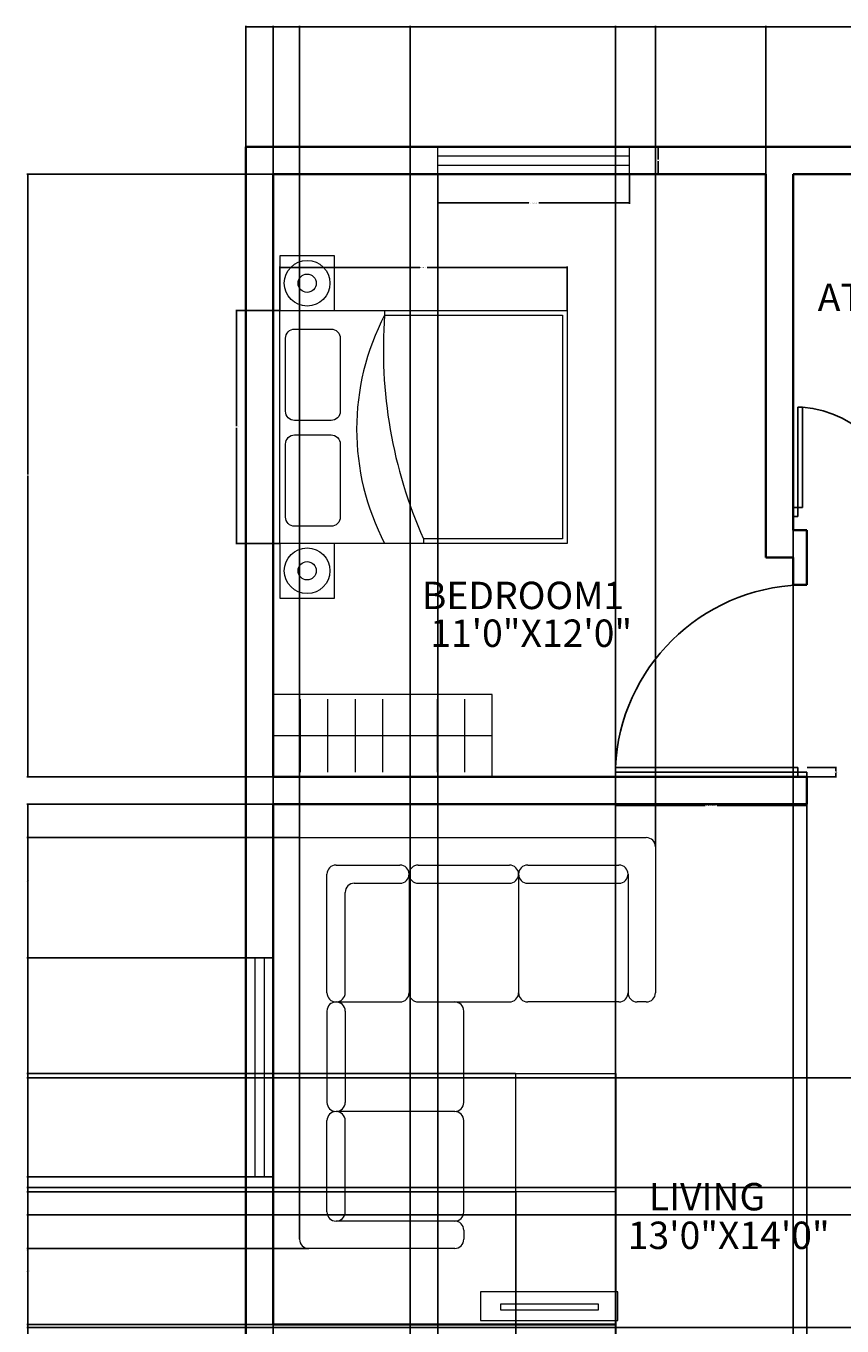
# Model space of a CAD drawing. Units: inches. Extents: x 2608 to 3003, y 1827 to 2396.
# Tile 3 of 5: x 2608 to 2787, y 2111 to 2396. Entities that reach past the tile are written whole.
import ezdxf

# ---------------------------------------------------------------- set-up
doc = ezdxf.new("R2010")
doc.units = ezdxf.units.IN
for name, color, linetype, lineweight in [('A-ANNO-DIMS', 2, 'Continuous', 18), ('A-AREA-IDEN', 7, 'Continuous', 25), ('A-DOOR', 50, 'Continuous', 25), ('A-EQPM', 213, 'Continuous', 18), ('A-FLOR-CASE', 213, 'Continuous', 18), ('A-FLOR-STRS', 111, 'Continuous', 25), ('A-FURN', 254, 'Continuous', 18), ('A-GLAZ', 40, 'Continuous', 18), ('A-WALL', 111, 'Continuous', 35)]:
    doc.layers.add(name, color=color, linetype=linetype, lineweight=lineweight)
doc.styles.get("Standard").update_dxf_attribs({"font": 'arial.ttf'})
doc.dimstyles.get("Standard").update_dxf_attribs({"dimtxt": 0.18, "dimasz": 0.18, "dimexe": 0.18, "dimexo": 0.0625, "dimgap": 0.09, "dimtad": 0, "dimtih": 1, "dimtoh": 1, "dimdec": 4, "dimzin": 0, "dimdsep": 46, "dimtxsty": 'Standard', "dimcen": 0.09, "dimadec": 0, "dimazin": 0, "dimtfac": 1, "dimtdec": 4, "dimtofl": 0, "dimtmove": 0, "dimatfit": 3, "dimfxl": 1, "dimtolj": 1, "dimtzin": 0, "dimarcsym": 0})

# ---------------------------------------------------------------- blocks, each defined once
blk = doc.blocks.new('BED-DOUBLE')
for p, q in [((22.99, 51), (22.99, 50)), ((22.99, 50), (61.99, 50)), ((61.99, 50), (61.99, 1)), ((61.99, 1), (31.5, 1)), ((31.5, 1), (31.5, 0))]:
    blk.add_line(p, q)
blk.add_lwpolyline([(0, 51), (63, 51), (63, 0), (0, 0)], close=True)
for points in [[(3.26, 46.94), (11.26, 46.94, -0.414214), (13.26, 44.94), (13.26, 28.94, -0.414214), (11.26, 26.94), (3.26, 26.94, -0.414214), (1.26, 28.94), (1.26, 44.94, -0.414214)], [(3.26, 23.76), (11.26, 23.76, -0.414214), (13.26, 21.76), (13.26, 5.76, -0.414214), (11.26, 3.76), (3.26, 3.76, -0.414214), (1.26, 5.76), (1.26, 21.76, -0.414214)]]:
    blk.add_lwpolyline(points, format="xyb", close=True)
for centre, radius, start, end in [((70.85, 25), 54, 152.4215, 207.5785), ((124.71, 42.43), 102, 175.743, 203.964)]:
    blk.add_arc(centre, radius, start, end)
blk = doc.blocks.new('NIGHTSTAND-LAMP')
blk.add_lwpolyline([(0, 0), (12, 0), (12, 12), (0, 12)], close=True)
for radius in [5, 2]:
    blk.add_circle((6, 6), radius)
blk = doc.blocks.new('WARDROBE-48')
for p, q in [((48, 18), (0, 18)), ((0, 18), (0, 0)), ((48, 0), (48, 18)), ((6, 1), (6, 17)), ((12, 1), (12, 17)), ((18, 1), (18, 17)), ((24, 1), (24, 17)), ((30, 1), (30, 17)), ((36, 1), (36, 17)), ((42, 1), (42, 17)), ((0, 9), (48, 9)), ((0, 0), (48, 0))]:
    blk.add_line(p, q)
blk = doc.blocks.new('WIN-42')
for p, q in [((0, 0), (0, 6)), ((42, 0), (42, 6)), ((0, 4), (42, 4)), ((0, 2), (42, 2))]:
    blk.add_line(p, q)
blk = doc.blocks.new('DOOR-LEAF-42')
for p, q in [((0, 1), (0, 2)), ((0, 2), (40, 2)), ((42, 1), (0, 1)), ((40, 2), (40, 0)), ((42, 0), (42, 1))]:
    blk.add_line(p, q)
blk = doc.blocks.new('*D14')
at = {"layer": 'A-ANNO-DIMS', "color": 0, "lineweight": -2, "transparency": 16777216}
for p, q in [((2663.35, 2333.66), (2663.35, 2343.23)), ((2663.53, 2343.05), (2694.03, 2343.05)), ((2726.17, 2343.05), (2695.67, 2343.05)), ((2726.35, 2333.66), (2726.35, 2343.23))]:
    blk.add_line(p, q, dxfattribs=at)
at = {"layer": 'A-ANNO-DIMS', "color": 0, "transparency": 16777216}
for points in [[(2663.53, 2343.08), (2663.53, 2343.02), (2663.35, 2343.05)], [(2726.17, 2343.08), (2726.17, 2343.02), (2726.35, 2343.05)]]:
    blk.add_solid(points, dxfattribs=at)
at = {"layer": 'Defpoints', "color": 0, "transparency": 16777216}
for p in [(2726.35, 2343.05), (2663.35, 2333.6), (2726.35, 2333.6)]:
    blk.add_point(p, dxfattribs=at)
at = {"layer": 'A-ANNO-DIMS', "color": 0, "transparency": 16777216, "insert": (2694.85, 2343.05), "char_height": 0.18, "attachment_point": 5}
blk.add_mtext('\\A1;BED 63 TYP.', dxfattribs=at)
blk = doc.blocks.new('*D15')
at = {"layer": 'A-ANNO-DIMS', "color": 0, "lineweight": -2, "transparency": 16777216}
for p, q in [((2663.29, 2333.6), (2653.72, 2333.6)), ((2653.9, 2333.42), (2653.9, 2308.28)), ((2653.9, 2282.78), (2653.9, 2307.92)), ((2663.29, 2282.6), (2653.72, 2282.6))]:
    blk.add_line(p, q, dxfattribs=at)
at = {"layer": 'A-ANNO-DIMS', "color": 0, "transparency": 16777216}
for points in [[(2653.87, 2333.42), (2653.93, 2333.42), (2653.9, 2333.6)], [(2653.87, 2282.78), (2653.93, 2282.78), (2653.9, 2282.6)]]:
    blk.add_solid(points, dxfattribs=at)
at = {"layer": 'Defpoints', "color": 0, "transparency": 16777216}
for p in [(2653.9, 2333.6), (2663.35, 2333.6), (2663.35, 2282.6)]:
    blk.add_point(p, dxfattribs=at)
at = {"layer": 'A-ANNO-DIMS', "color": 0, "transparency": 16777216, "insert": (2653.9, 2308.1), "char_height": 0.18, "attachment_point": 5}
blk.add_mtext('\\A1;51 TYP.', dxfattribs=at)
blk = doc.blocks.new('*D22')
at = {"layer": 'A-ANNO-DIMS', "color": 0, "lineweight": -2, "transparency": 16777216}
for p, q in [((2698.03, 2363.43), (2698.03, 2357.01)), ((2740.03, 2363.43), (2740.03, 2357.01)), ((2698.21, 2357.19), (2717.91, 2357.19)), ((2739.85, 2357.19), (2720.15, 2357.19))]:
    blk.add_line(p, q, dxfattribs=at)
at = {"layer": 'A-ANNO-DIMS', "color": 0, "transparency": 16777216}
for points in [[(2698.21, 2357.22), (2698.21, 2357.16), (2698.03, 2357.19)], [(2739.85, 2357.22), (2739.85, 2357.16), (2740.03, 2357.19)]]:
    blk.add_solid(points, dxfattribs=at)
at = {"layer": 'Defpoints', "color": 0, "transparency": 16777216}
for p in [(2698.03, 2363.49), (2740.03, 2363.49), (2740.03, 2357.19)]:
    blk.add_point(p, dxfattribs=at)
at = {"layer": 'A-ANNO-DIMS', "color": 0, "transparency": 16777216, "insert": (2719.03, 2357.19), "char_height": 0.18, "attachment_point": 5}
blk.add_mtext('\\A1;WINDOW 42 TYP.', dxfattribs=at)
blk = doc.blocks.new('*D23')
at = {"layer": 'A-ANNO-DIMS', "color": 0, "lineweight": -2, "transparency": 16777216}
for p, q in [((2740.09, 2369.49), (2746.51, 2369.49)), ((2746.33, 2369.31), (2746.33, 2366.67)), ((2746.33, 2363.67), (2746.33, 2366.31)), ((2740.09, 2363.49), (2746.51, 2363.49))]:
    blk.add_line(p, q, dxfattribs=at)
at = {"layer": 'A-ANNO-DIMS', "color": 0, "transparency": 16777216}
for points in [[(2746.3, 2369.31), (2746.36, 2369.31), (2746.33, 2369.49)], [(2746.3, 2363.67), (2746.36, 2363.67), (2746.33, 2363.49)]]:
    blk.add_solid(points, dxfattribs=at)
at = {"layer": 'Defpoints', "color": 0, "transparency": 16777216}
for p in [(2740.03, 2369.49), (2746.33, 2369.49), (2740.03, 2363.49)]:
    blk.add_point(p, dxfattribs=at)
at = {"layer": 'A-ANNO-DIMS', "color": 0, "transparency": 16777216, "insert": (2746.33, 2366.49), "char_height": 0.18, "attachment_point": 5}
blk.add_mtext('\\A1;6 TYP.', dxfattribs=at)
blk = doc.blocks.new('*D24')
at = {"layer": 'A-ANNO-DIMS', "color": 0, "lineweight": -2, "transparency": 16777216}
for p, q in [((2736.92, 2231.43), (2736.92, 2225.01)), ((2778.92, 2231.43), (2778.92, 2225.01)), ((2737.1, 2225.19), (2756.63, 2225.19)), ((2778.74, 2225.19), (2759.2, 2225.19))]:
    blk.add_line(p, q, dxfattribs=at)
at = {"layer": 'A-ANNO-DIMS', "color": 0, "transparency": 16777216}
for points in [[(2737.1, 2225.22), (2737.1, 2225.16), (2736.92, 2225.19)], [(2778.74, 2225.22), (2778.74, 2225.16), (2778.92, 2225.19)]]:
    blk.add_solid(points, dxfattribs=at)
at = {"layer": 'Defpoints', "color": 0, "transparency": 16777216}
for p in [(2736.92, 2231.49), (2778.92, 2231.49), (2778.92, 2225.19)]:
    blk.add_point(p, dxfattribs=at)
at = {"layer": 'A-ANNO-DIMS', "color": 0, "transparency": 16777216, "insert": (2757.92, 2225.19), "char_height": 0.18, "attachment_point": 5}
blk.add_mtext('\\A1;DOOR LEAF 42 TYP.', dxfattribs=at)
blk = doc.blocks.new('*D25')
at = {"layer": 'A-ANNO-DIMS', "color": 0, "lineweight": -2, "transparency": 16777216}
for p, q in [((2778.98, 2233.49), (2785.4, 2233.49)), ((2785.22, 2233.31), (2785.22, 2232.67)), ((2778.98, 2231.49), (2785.4, 2231.49)), ((2785.22, 2231.67), (2785.22, 2232.31))]:
    blk.add_line(p, q, dxfattribs=at)
at = {"layer": 'A-ANNO-DIMS', "color": 0, "transparency": 16777216}
for points in [[(2785.19, 2233.31), (2785.25, 2233.31), (2785.22, 2233.49)], [(2785.19, 2231.67), (2785.25, 2231.67), (2785.22, 2231.49)]]:
    blk.add_solid(points, dxfattribs=at)
at = {"layer": 'Defpoints', "color": 0, "transparency": 16777216}
for p in [(2778.92, 2233.49), (2785.22, 2233.49), (2778.92, 2231.49)]:
    blk.add_point(p, dxfattribs=at)
at = {"layer": 'A-ANNO-DIMS', "color": 0, "transparency": 16777216, "insert": (2785.22, 2232.49), "char_height": 0.18, "attachment_point": 5}
blk.add_mtext('\\A1;2 TYP.', dxfattribs=at)
blk = doc.blocks.new('*D28')
at = {"layer": 'A-ANNO-DIMS', "color": 0, "lineweight": -2, "transparency": 16777216}
for p, q in [((2655.92, 2191.9), (2655.92, 2395.95)), ((2656.1, 2395.77), (2805.63, 2395.77)), ((2955.74, 2395.77), (2806.2, 2395.77)), ((2955.92, 2201.05), (2955.92, 2395.95))]:
    blk.add_line(p, q, dxfattribs=at)
at = {"layer": 'A-ANNO-DIMS', "color": 0, "transparency": 16777216}
for points in [[(2656.1, 2395.8), (2656.1, 2395.74), (2655.92, 2395.77)], [(2955.74, 2395.8), (2955.74, 2395.74), (2955.92, 2395.77)]]:
    blk.add_solid(points, dxfattribs=at)
at = {"layer": 'Defpoints', "color": 0, "transparency": 16777216}
for p in [(2955.92, 2395.77), (2955.92, 2200.98), (2655.92, 2191.84)]:
    blk.add_point(p, dxfattribs=at)
at = {"layer": 'A-ANNO-DIMS', "color": 0, "transparency": 16777216, "insert": (2805.92, 2395.77), "char_height": 0.18, "attachment_point": 5}
blk.add_mtext('\\A1;300', dxfattribs=at)
blk = doc.blocks.new('*D35')
at = {"layer": 'A-ANNO-DIMS', "color": 0, "lineweight": -2, "transparency": 16777216}
for p, q in [((2661.85, 2143.84), (2607.92, 2143.84)), ((2608.1, 2143.66), (2608.1, 2127.85)), ((2608.1, 2111.67), (2608.1, 2127.48)), ((2661.85, 2111.49), (2607.92, 2111.49))]:
    blk.add_line(p, q, dxfattribs=at)
at = {"layer": 'A-ANNO-DIMS', "color": 0, "transparency": 16777216}
for points in [[(2608.07, 2143.66), (2608.13, 2143.66), (2608.1, 2143.84)], [(2608.07, 2111.67), (2608.13, 2111.67), (2608.1, 2111.49)]]:
    blk.add_solid(points, dxfattribs=at)
at = {"layer": 'Defpoints', "color": 0, "transparency": 16777216}
for p in [(2608.1, 2143.84), (2661.92, 2143.84), (2661.92, 2111.49)]:
    blk.add_point(p, dxfattribs=at)
at = {"layer": 'A-ANNO-DIMS', "color": 0, "transparency": 16777216, "insert": (2608.1, 2127.66), "char_height": 0.18, "attachment_point": 5}
blk.add_mtext('\\A1;32.35', dxfattribs=at)
blk = doc.blocks.new('*D36')
at = {"layer": 'A-ANNO-DIMS', "color": 0, "lineweight": -2, "transparency": 16777216}
for p, q in [((2655.85, 2191.84), (2607.92, 2191.84)), ((2608.1, 2191.66), (2608.1, 2168.02)), ((2608.1, 2144.02), (2608.1, 2167.66)), ((2655.85, 2143.84), (2607.92, 2143.84))]:
    blk.add_line(p, q, dxfattribs=at)
at = {"layer": 'A-ANNO-DIMS', "color": 0, "transparency": 16777216}
for points in [[(2608.07, 2191.66), (2608.13, 2191.66), (2608.1, 2191.84)], [(2608.07, 2144.02), (2608.13, 2144.02), (2608.1, 2143.84)]]:
    blk.add_solid(points, dxfattribs=at)
at = {"layer": 'Defpoints', "color": 0, "transparency": 16777216}
for p in [(2608.1, 2191.84), (2655.92, 2191.84), (2655.92, 2143.84)]:
    blk.add_point(p, dxfattribs=at)
at = {"layer": 'A-ANNO-DIMS', "color": 0, "transparency": 16777216, "insert": (2608.1, 2167.84), "char_height": 0.18, "attachment_point": 5}
blk.add_mtext('\\A1;48', dxfattribs=at)
blk = doc.blocks.new('*D37')
at = {"layer": 'A-ANNO-DIMS', "color": 0, "lineweight": -2, "transparency": 16777216}
for p, q in [((2661.85, 2225.49), (2607.92, 2225.49)), ((2608.1, 2225.31), (2608.1, 2208.85)), ((2608.1, 2192.02), (2608.1, 2208.48)), ((2661.85, 2191.84), (2607.92, 2191.84))]:
    blk.add_line(p, q, dxfattribs=at)
at = {"layer": 'A-ANNO-DIMS', "color": 0, "transparency": 16777216}
for points in [[(2608.07, 2225.31), (2608.13, 2225.31), (2608.1, 2225.49)], [(2608.07, 2192.02), (2608.13, 2192.02), (2608.1, 2191.84)]]:
    blk.add_solid(points, dxfattribs=at)
at = {"layer": 'Defpoints', "color": 0, "transparency": 16777216}
for p in [(2608.1, 2225.49), (2661.92, 2225.49), (2661.92, 2191.84)]:
    blk.add_point(p, dxfattribs=at)
at = {"layer": 'A-ANNO-DIMS', "color": 0, "transparency": 16777216, "insert": (2608.1, 2208.66), "char_height": 0.18, "attachment_point": 5}
blk.add_mtext('\\A1;33.65', dxfattribs=at)
blk = doc.blocks.new('*D38')
at = {"layer": 'A-ANNO-DIMS', "color": 0, "lineweight": -2, "transparency": 16777216}
for p, q in [((2661.92, 2363.55), (2661.92, 2395.95)), ((2662.1, 2395.77), (2715.63, 2395.77)), ((2769.74, 2395.77), (2716.2, 2395.77)), ((2769.92, 2363.55), (2769.92, 2395.95))]:
    blk.add_line(p, q, dxfattribs=at)
at = {"layer": 'A-ANNO-DIMS', "color": 0, "transparency": 16777216}
for points in [[(2662.1, 2395.8), (2662.1, 2395.74), (2661.92, 2395.77)], [(2769.74, 2395.8), (2769.74, 2395.74), (2769.92, 2395.77)]]:
    blk.add_solid(points, dxfattribs=at)
at = {"layer": 'Defpoints', "color": 0, "transparency": 16777216}
for p in [(2769.92, 2395.77), (2661.92, 2363.49), (2769.92, 2363.49)]:
    blk.add_point(p, dxfattribs=at)
at = {"layer": 'A-ANNO-DIMS', "color": 0, "transparency": 16777216, "insert": (2715.92, 2395.77), "char_height": 0.18, "attachment_point": 5}
blk.add_mtext('\\A1;108', dxfattribs=at)
blk = doc.blocks.new('*D40')
at = {"layer": 'A-ANNO-DIMS', "color": 0, "lineweight": -2, "transparency": 16777216}
for p, q in [((2661.85, 2363.49), (2607.92, 2363.49)), ((2608.1, 2363.31), (2608.1, 2297.67)), ((2608.1, 2231.67), (2608.1, 2297.31)), ((2661.85, 2231.49), (2607.92, 2231.49))]:
    blk.add_line(p, q, dxfattribs=at)
at = {"layer": 'A-ANNO-DIMS', "color": 0, "transparency": 16777216}
for points in [[(2608.07, 2363.31), (2608.13, 2363.31), (2608.1, 2363.49)], [(2608.07, 2231.67), (2608.13, 2231.67), (2608.1, 2231.49)]]:
    blk.add_solid(points, dxfattribs=at)
at = {"layer": 'Defpoints', "color": 0, "transparency": 16777216}
for p in [(2608.1, 2363.49), (2661.92, 2363.49), (2661.92, 2231.49)]:
    blk.add_point(p, dxfattribs=at)
at = {"layer": 'A-ANNO-DIMS', "color": 0, "transparency": 16777216, "insert": (2608.1, 2297.49), "char_height": 0.18, "attachment_point": 5}
blk.add_mtext('\\A1;132', dxfattribs=at)
blk = doc.blocks.new('*D42')
at = {"layer": 'A-ANNO-DIMS', "color": 0, "lineweight": -2, "transparency": 16777216}
for p, q in [((2775.92, 2285.43), (2775.92, 1827.03)), ((2799.92, 2285.43), (2799.92, 1827.03)), ((2776.1, 1827.21), (2787.7, 1827.21)), ((2799.74, 1827.21), (2788.14, 1827.21))]:
    blk.add_line(p, q, dxfattribs=at)
at = {"layer": 'A-ANNO-DIMS', "color": 0, "transparency": 16777216}
for points in [[(2776.1, 1827.24), (2776.1, 1827.18), (2775.92, 1827.21)], [(2799.74, 1827.24), (2799.74, 1827.18), (2799.92, 1827.21)]]:
    blk.add_solid(points, dxfattribs=at)
at = {"layer": 'Defpoints', "color": 0, "transparency": 16777216}
for p in [(2775.92, 2285.49), (2799.92, 2285.49), (2799.92, 1827.21)]:
    blk.add_point(p, dxfattribs=at)
at = {"layer": 'A-ANNO-DIMS', "color": 0, "transparency": 16777216, "insert": (2787.92, 1827.21), "char_height": 0.18, "attachment_point": 5}
blk.add_mtext('\\A1;24', dxfattribs=at)
blk = doc.blocks.new('*D43')
at = {"layer": 'A-ANNO-DIMS', "color": 0, "lineweight": -2, "transparency": 16777216}
for p, q in [((2661.92, 2363.43), (2661.92, 1827.03)), ((2698.03, 2363.43), (2698.03, 1827.03)), ((2662.1, 1827.21), (2679.51, 1827.21)), ((2697.85, 1827.21), (2680.44, 1827.21))]:
    blk.add_line(p, q, dxfattribs=at)
at = {"layer": 'A-ANNO-DIMS', "color": 0, "transparency": 16777216}
for points in [[(2662.1, 1827.24), (2662.1, 1827.18), (2661.92, 1827.21)], [(2697.85, 1827.24), (2697.85, 1827.18), (2698.03, 1827.21)]]:
    blk.add_solid(points, dxfattribs=at)
at = {"layer": 'Defpoints', "color": 0, "transparency": 16777216}
for p in [(2661.92, 2363.49), (2698.03, 2363.49), (2698.03, 1827.21)]:
    blk.add_point(p, dxfattribs=at)
at = {"layer": 'A-ANNO-DIMS', "color": 0, "transparency": 16777216, "insert": (2679.97, 1827.21), "char_height": 0.18, "attachment_point": 5}
blk.add_mtext('\\A1;36.116', dxfattribs=at)
blk = doc.blocks.new('*D44')
at = {"layer": 'A-ANNO-DIMS', "color": 0, "lineweight": -2, "transparency": 16777216}
for p, q in [((2775.92, 2363.43), (2775.92, 1827.03)), ((2795.68, 2363.43), (2795.68, 1827.03)), ((2776.1, 1827.21), (2785.34, 1827.21)), ((2795.5, 1827.21), (2786.25, 1827.21))]:
    blk.add_line(p, q, dxfattribs=at)
at = {"layer": 'A-ANNO-DIMS', "color": 0, "transparency": 16777216}
for points in [[(2776.1, 1827.24), (2776.1, 1827.18), (2775.92, 1827.21)], [(2795.5, 1827.24), (2795.5, 1827.18), (2795.68, 1827.21)]]:
    blk.add_solid(points, dxfattribs=at)
at = {"layer": 'Defpoints', "color": 0, "transparency": 16777216}
for p in [(2775.92, 2363.49), (2795.68, 2363.49), (2795.68, 1827.21)]:
    blk.add_point(p, dxfattribs=at)
at = {"layer": 'A-ANNO-DIMS', "color": 0, "transparency": 16777216, "insert": (2785.8, 1827.21), "char_height": 0.18, "attachment_point": 5}
blk.add_mtext('\\A1;19.766', dxfattribs=at)
blk = doc.blocks.new('*D47')
at = {"layer": 'A-ANNO-DIMS', "color": 0, "lineweight": -2, "transparency": 16777216}
for p, q in [((2778.92, 2225.43), (2778.92, 1827.03)), ((2835.92, 2225.43), (2835.92, 1827.03)), ((2779.1, 1827.21), (2807.2, 1827.21)), ((2835.74, 1827.21), (2807.63, 1827.21))]:
    blk.add_line(p, q, dxfattribs=at)
at = {"layer": 'A-ANNO-DIMS', "color": 0, "transparency": 16777216}
for points in [[(2779.1, 1827.24), (2779.1, 1827.18), (2778.92, 1827.21)], [(2835.74, 1827.24), (2835.74, 1827.18), (2835.92, 1827.21)]]:
    blk.add_solid(points, dxfattribs=at)
at = {"layer": 'Defpoints', "color": 0, "transparency": 16777216}
for p in [(2778.92, 2225.49), (2835.92, 2225.49), (2835.92, 1827.21)]:
    blk.add_point(p, dxfattribs=at)
at = {"layer": 'A-ANNO-DIMS', "color": 0, "transparency": 16777216, "insert": (2807.42, 1827.21), "char_height": 0.18, "attachment_point": 5}
blk.add_mtext('\\A1;57', dxfattribs=at)
blk = doc.blocks.new('*D48')
at = {"layer": 'A-ANNO-DIMS', "color": 0, "lineweight": -2, "transparency": 16777216}
for p, q in [((2889.85, 2165.49), (2607.92, 2165.49)), ((2608.1, 2165.31), (2608.1, 2153.67)), ((2608.1, 2141.67), (2608.1, 2153.31)), ((2889.85, 2141.49), (2607.92, 2141.49))]:
    blk.add_line(p, q, dxfattribs=at)
at = {"layer": 'A-ANNO-DIMS', "color": 0, "transparency": 16777216}
for points in [[(2608.07, 2165.31), (2608.13, 2165.31), (2608.1, 2165.49)], [(2608.07, 2141.67), (2608.13, 2141.67), (2608.1, 2141.49)]]:
    blk.add_solid(points, dxfattribs=at)
at = {"layer": 'Defpoints', "color": 0, "transparency": 16777216}
for p in [(2608.1, 2165.49), (2889.92, 2165.49), (2889.92, 2141.49)]:
    blk.add_point(p, dxfattribs=at)
at = {"layer": 'A-ANNO-DIMS', "color": 0, "transparency": 16777216, "insert": (2608.1, 2153.49), "char_height": 0.18, "attachment_point": 5}
blk.add_mtext('\\A1;24', dxfattribs=at)
blk = doc.blocks.new('*D55')
at = {"layer": 'A-ANNO-DIMS', "color": 0, "lineweight": -2, "transparency": 16777216}
for p, q in [((2847.85, 2135.49), (2607.92, 2135.49)), ((2608.1, 2135.31), (2608.1, 2122.17)), ((2608.1, 2108.67), (2608.1, 2121.81)), ((2853.85, 2108.49), (2607.92, 2108.49))]:
    blk.add_line(p, q, dxfattribs=at)
at = {"layer": 'A-ANNO-DIMS', "color": 0, "transparency": 16777216}
for points in [[(2608.07, 2135.31), (2608.13, 2135.31), (2608.1, 2135.49)], [(2608.07, 2108.67), (2608.13, 2108.67), (2608.1, 2108.49)]]:
    blk.add_solid(points, dxfattribs=at)
at = {"layer": 'Defpoints', "color": 0, "transparency": 16777216}
for p in [(2608.1, 2135.49), (2847.92, 2135.49), (2853.92, 2108.49)]:
    blk.add_point(p, dxfattribs=at)
at = {"layer": 'A-ANNO-DIMS', "color": 0, "transparency": 16777216, "insert": (2608.1, 2121.99), "char_height": 0.18, "attachment_point": 5}
blk.add_mtext('\\A1;27', dxfattribs=at)
blk = doc.blocks.new('*D62')
at = {"layer": 'A-ANNO-DIMS', "color": 0, "lineweight": -2, "transparency": 16777216}
for p, q in [((2925.85, 2135.49), (2607.92, 2135.49)), ((2608.1, 2135.31), (2608.1, 2123.33)), ((2608.1, 2110.99), (2608.1, 2122.97)), ((2928.1, 2110.81), (2607.92, 2110.81))]:
    blk.add_line(p, q, dxfattribs=at)
at = {"layer": 'A-ANNO-DIMS', "color": 0, "transparency": 16777216}
for points in [[(2608.07, 2135.31), (2608.13, 2135.31), (2608.1, 2135.49)], [(2608.07, 2110.99), (2608.13, 2110.99), (2608.1, 2110.81)]]:
    blk.add_solid(points, dxfattribs=at)
at = {"layer": 'Defpoints', "color": 0, "transparency": 16777216}
for p in [(2925.92, 2135.49), (2608.1, 2110.81), (2928.16, 2110.81)]:
    blk.add_point(p, dxfattribs=at)
at = {"layer": 'A-ANNO-DIMS', "color": 0, "transparency": 16777216, "insert": (2608.1, 2123.15), "char_height": 0.18, "attachment_point": 5}
blk.add_mtext('\\A1;24.675', dxfattribs=at)
blk = doc.blocks.new('*D69')
at = {"layer": 'A-ANNO-DIMS', "color": 0, "lineweight": -2, "transparency": 16777216}
for p, q in [((2691.92, 2105.55), (2691.92, 2395.95)), ((2692.1, 2395.77), (2714.19, 2395.77)), ((2736.74, 2395.77), (2714.64, 2395.77)), ((2736.92, 2105.55), (2736.92, 2395.95))]:
    blk.add_line(p, q, dxfattribs=at)
at = {"layer": 'A-ANNO-DIMS', "color": 0, "transparency": 16777216}
for points in [[(2692.1, 2395.8), (2692.1, 2395.74), (2691.92, 2395.77)], [(2736.74, 2395.8), (2736.74, 2395.74), (2736.92, 2395.77)]]:
    blk.add_solid(points, dxfattribs=at)
at = {"layer": 'Defpoints', "color": 0, "transparency": 16777216}
for p in [(2736.92, 2395.77), (2691.92, 2105.49), (2736.92, 2105.49)]:
    blk.add_point(p, dxfattribs=at)
at = {"layer": 'A-ANNO-DIMS', "color": 0, "transparency": 16777216, "insert": (2714.42, 2395.77), "char_height": 0.18, "attachment_point": 5}
blk.add_mtext('\\A1;45', dxfattribs=at)
blk = doc.blocks.new('*D72')
at = {"layer": 'A-ANNO-DIMS', "color": 0, "lineweight": -2, "transparency": 16777216}
for p, q in [((2715.11, 2140.45), (2715.11, 1827.03)), ((2737, 2140.45), (2737, 1827.03)), ((2715.29, 1827.21), (2725.66, 1827.21)), ((2736.82, 1827.21), (2726.45, 1827.21))]:
    blk.add_line(p, q, dxfattribs=at)
at = {"layer": 'A-ANNO-DIMS', "color": 0, "transparency": 16777216}
for points in [[(2715.29, 1827.24), (2715.29, 1827.18), (2715.11, 1827.21)], [(2736.82, 1827.24), (2736.82, 1827.18), (2737, 1827.21)]]:
    blk.add_solid(points, dxfattribs=at)
at = {"layer": 'Defpoints', "color": 0, "transparency": 16777216}
for p in [(2715.11, 2140.51), (2737, 2140.51), (2737, 1827.21)]:
    blk.add_point(p, dxfattribs=at)
at = {"layer": 'A-ANNO-DIMS', "color": 0, "transparency": 16777216, "insert": (2726.06, 1827.21), "char_height": 0.18, "attachment_point": 5}
blk.add_mtext('\\A1;21.89', dxfattribs=at)
blk = doc.blocks.new('*D73')
at = {"layer": 'A-ANNO-DIMS', "color": 0, "lineweight": -2, "transparency": 16777216}
for p, q in [((2715.05, 2166.47), (2607.92, 2166.47)), ((2608.1, 2166.29), (2608.1, 2153.67)), ((2608.1, 2140.69), (2608.1, 2153.31)), ((2715.05, 2140.51), (2607.92, 2140.51))]:
    blk.add_line(p, q, dxfattribs=at)
at = {"layer": 'A-ANNO-DIMS', "color": 0, "transparency": 16777216}
for points in [[(2608.07, 2166.29), (2608.13, 2166.29), (2608.1, 2166.47)], [(2608.07, 2140.69), (2608.13, 2140.69), (2608.1, 2140.51)]]:
    blk.add_solid(points, dxfattribs=at)
at = {"layer": 'Defpoints', "color": 0, "transparency": 16777216}
for p in [(2608.1, 2166.47), (2715.11, 2166.47), (2715.11, 2140.51)]:
    blk.add_point(p, dxfattribs=at)
at = {"layer": 'A-ANNO-DIMS', "color": 0, "transparency": 16777216, "insert": (2608.1, 2153.49), "char_height": 0.18, "attachment_point": 5}
blk.add_mtext('\\A1;25.96', dxfattribs=at)
blk = doc.blocks.new('*D74')
at = {"layer": 'A-ANNO-DIMS', "color": 0, "lineweight": -2, "transparency": 16777216}
for p, q in [((2667.69, 2130.21), (2667.69, 2395.95)), ((2667.87, 2395.77), (2706.47, 2395.77)), ((2745.51, 2395.77), (2706.91, 2395.77)), ((2745.69, 2216.21), (2745.69, 2395.95))]:
    blk.add_line(p, q, dxfattribs=at)
at = {"layer": 'A-ANNO-DIMS', "color": 0, "transparency": 16777216}
for points in [[(2667.87, 2395.8), (2667.87, 2395.74), (2667.69, 2395.77)], [(2745.51, 2395.8), (2745.51, 2395.74), (2745.69, 2395.77)]]:
    blk.add_solid(points, dxfattribs=at)
at = {"layer": 'Defpoints', "color": 0, "transparency": 16777216}
for p in [(2745.69, 2395.77), (2745.69, 2216.14), (2667.69, 2130.14)]:
    blk.add_point(p, dxfattribs=at)
at = {"layer": 'A-ANNO-DIMS', "color": 0, "transparency": 16777216, "insert": (2706.69, 2395.77), "char_height": 0.18, "attachment_point": 5}
blk.add_mtext('\\A1;78', dxfattribs=at)
blk = doc.blocks.new('*D75')
at = {"layer": 'A-ANNO-DIMS', "color": 0, "lineweight": -2, "transparency": 16777216}
for p, q in [((2667.63, 2218.14), (2607.92, 2218.14)), ((2608.1, 2217.96), (2608.1, 2173.32)), ((2608.1, 2128.32), (2608.1, 2172.96)), ((2669.63, 2128.14), (2607.92, 2128.14))]:
    blk.add_line(p, q, dxfattribs=at)
at = {"layer": 'A-ANNO-DIMS', "color": 0, "transparency": 16777216}
for points in [[(2608.07, 2217.96), (2608.13, 2217.96), (2608.1, 2218.14)], [(2608.07, 2128.32), (2608.13, 2128.32), (2608.1, 2128.14)]]:
    blk.add_solid(points, dxfattribs=at)
at = {"layer": 'Defpoints', "color": 0, "transparency": 16777216}
for p in [(2608.1, 2218.14), (2667.69, 2218.14), (2669.69, 2128.14)]:
    blk.add_point(p, dxfattribs=at)
at = {"layer": 'A-ANNO-DIMS', "color": 0, "transparency": 16777216, "insert": (2608.1, 2173.14), "char_height": 0.18, "attachment_point": 5}
blk.add_mtext('\\A1;90', dxfattribs=at)
blk = doc.blocks.new('*D76')
at = {"layer": 'A-ANNO-DIMS', "color": 0, "lineweight": -2, "transparency": 16777216}
for p, q in [((2813.16, 2112.32), (2794.82, 2095.3)), ((2813.34, 2112.32), (2813.16, 2112.32)), ((2763.83, 2066.6), (2764.01, 2066.6)), ((2763.92, 2066.51), (2763.92, 2066.69))]:
    blk.add_line(p, q, dxfattribs=at)
at = {"layer": 'A-ANNO-DIMS', "color": 0, "transparency": 16777216}
blk.add_solid([(2794.8, 2095.32), (2794.85, 2095.28), (2794.69, 2095.18)], dxfattribs=at)
at = {"layer": 'Defpoints', "color": 0, "transparency": 16777216}
for p in [(2794.69, 2095.18), (2763.92, 2066.6)]:
    blk.add_point(p, dxfattribs=at)
at = {"layer": 'A-ANNO-DIMS', "color": 0, "transparency": 16777216, "insert": (2813.64, 2112.32), "char_height": 0.18, "attachment_point": 5}
blk.add_mtext('\\A1;R42', dxfattribs=at)

msp = doc.modelspace()

# ---------------------------------------------------------------- linework, layer by layer
at = {"layer": 'A-DOOR'}
for p, q in [((2776.9155, 2288.4603), (2776.9155, 2312.4603)), ((2776.9155, 2312.4603), (2777.9155, 2312.4603)), ((2777.9155, 2312.4603), (2777.9155, 2290.4603)), ((2777.9155, 2290.4603), (2775.9155, 2290.4603)), ((2775.9155, 2288.4603), (2776.9155, 2288.4603))]:
    msp.add_line(p, q, dxfattribs=at)
for centre, radius, start, end in [((2775.9156, 2288.5438), 24, 359.870639, 85.219955), ((2778.8691, 2231.5148), 42, 91.983302, 177.304959)]:
    msp.add_arc(centre, radius, start, end, dxfattribs=at)
at = {"layer": 'A-EQPM'}
for points in [[(2707.3148, 2112.3224), (2737.4539, 2112.3224), (2737.4539, 2118.6043), (2707.3148, 2118.6043)], [(2711.7858, 2115.998), (2733.1602, 2115.998), (2733.1602, 2114.593), (2711.7858, 2114.593)]]:
    msp.add_lwpolyline(points, close=True, dxfattribs=at)
at = {"layer": 'A-FLOR-CASE'}
msp.add_line((2661.9155, 2231.4896), (2661.9155, 2249.4896), dxfattribs=at)
at = {"layer": 'A-FLOR-STRS'}
msp.add_line((2736.9155, 2067.4896), (2736.9155, 2111.4896), dxfattribs=at)
at = {"layer": 'A-FURN'}
for p, q in [((2667.6933, 2218.1429), (2743.6933, 2218.1429)), ((2667.6933, 2182.1429), (2667.6933, 2218.1429)), ((2745.6933, 2216.1429), (2745.6933, 2184.1429)), ((2673.6933, 2184.1429), (2673.6933, 2210.1429)), ((2675.6933, 2212.1429), (2689.6933, 2212.1429)), ((2691.6933, 2210.1429), (2691.6933, 2210.1429)), ((2691.6933, 2210.1429), (2691.6933, 2210.1429)), ((2691.6933, 2210.1429), (2691.6933, 2184.1429)), ((2693.6933, 2212.1429), (2713.6933, 2212.1429)), ((2715.6933, 2210.1429), (2715.6933, 2210.1429)), ((2715.6933, 2210.1429), (2715.6933, 2210.1429)), ((2715.6933, 2210.1429), (2715.6933, 2184.1429)), ((2717.6933, 2212.1429), (2737.6933, 2212.1429)), ((2739.6933, 2210.1429), (2739.6933, 2210.1429)), ((2739.6933, 2210.1429), (2739.6933, 2184.1429)), ((2679.6933, 2208.1429), (2689.6933, 2208.1429)), ((2693.6933, 2208.1429), (2713.6933, 2208.1429)), ((2717.6933, 2208.1429), (2737.6933, 2208.1429)), ((2677.6933, 2184.1429), (2677.6933, 2206.1429)), ((2667.6933, 2130.1429), (2667.6933, 2182.1429)), ((2675.6933, 2182.1429), (2675.6933, 2182.1429)), ((2675.6933, 2182.1429), (2675.6933, 2182.1429)), ((2675.6933, 2182.1429), (2689.6933, 2182.1429)), ((2691.6933, 2184.1429), (2691.6933, 2184.1429)), ((2693.6933, 2182.1429), (2701.6933, 2182.1429)), ((2701.6933, 2182.1429), (2713.6933, 2182.1429)), ((2715.6933, 2184.1429), (2715.6933, 2184.1429)), ((2737.6933, 2182.1429), (2717.6933, 2182.1429)), ((2739.6933, 2184.1429), (2739.6933, 2184.1429)), ((2743.6933, 2182.1429), (2741.6933, 2182.1429)), ((2673.6933, 2180.1429), (2673.6933, 2160.1429)), ((2677.6933, 2180.1429), (2677.6933, 2160.1429)), ((2703.6933, 2160.1429), (2703.6933, 2180.1429)), ((2673.6933, 2136.1429), (2673.6933, 2156.1429)), ((2675.6933, 2158.1429), (2675.6933, 2158.1429)), ((2675.6933, 2158.1429), (2675.6933, 2158.1429)), ((2701.6933, 2158.1429), (2675.6933, 2158.1429)), ((2677.6933, 2136.1429), (2677.6933, 2156.1429)), ((2701.6933, 2158.1429), (2701.6933, 2158.1429)), ((2703.6933, 2136.1429), (2703.6933, 2156.1429)), ((2675.6933, 2134.1429), (2675.6933, 2134.1429)), ((2701.6933, 2134.1429), (2675.6933, 2134.1429)), ((2701.6933, 2134.1429), (2701.6933, 2134.1429)), ((2703.6933, 2132.1429), (2703.6933, 2130.1429)), ((2701.6933, 2128.1429), (2669.6933, 2128.1429))]:
    msp.add_line(p, q, dxfattribs=at)
msp.add_lwpolyline([(2715.1137, 2166.4712), (2737.0038, 2166.4712), (2737.0038, 2140.51), (2715.1137, 2140.51)], close=True, dxfattribs=at)
for centre, start, end in [((2743.6933, 2216.1429), 0, 90), ((2675.6933, 2210.1429), 90, 180), ((2689.6933, 2210.1429), 360, 90), ((2689.6933, 2210.1429), 270, 360), ((2693.6933, 2210.1429), 90, 180), ((2693.6933, 2210.1429), 180, 270), ((2713.6933, 2210.1429), 0, 90), ((2713.6933, 2210.1429), 270, 0), ((2717.6933, 2210.1429), 90, 180), ((2717.6933, 2210.1429), 180, 270), ((2737.6933, 2210.1429), 0, 90), ((2737.6933, 2210.1429), 270, 0), ((2679.6933, 2206.1429), 90, 180), ((2675.6933, 2184.1429), 180, 270), ((2675.6933, 2180.1429), 90, 180), ((2675.6933, 2184.1429), 270, 0), ((2675.6933, 2180.1429), 0, 90), ((2689.6933, 2184.1429), 270, 0), ((2693.6933, 2184.1429), 180, 270), ((2701.6933, 2180.1429), 0, 90), ((2713.6933, 2184.1429), 270, 0), ((2717.6933, 2184.1429), 180, 270), ((2737.6933, 2184.1429), 270, 0), ((2741.6933, 2184.1429), 180, 270), ((2743.6933, 2184.1429), 270, 0), ((2675.6933, 2160.1429), 180, 270), ((2675.6933, 2160.1429), 270, 0), ((2701.6933, 2160.1429), 270, 0), ((2675.6933, 2156.1429), 90, 180), ((2675.6933, 2156.1429), 0, 90), ((2701.6933, 2156.1429), 0, 90), ((2675.6933, 2136.1429), 180, 270), ((2675.6933, 2136.1429), 270, 0), ((2701.6933, 2136.1429), 270, 0), ((2701.6933, 2132.1429), 0, 90), ((2669.6933, 2130.1429), 180, 270), ((2701.6933, 2130.1429), 270, 0)]:
    msp.add_arc(centre, 2, start, end, dxfattribs=at)
at = {"layer": 'A-GLAZ'}
for p, q in [((2661.9155, 2191.8395), (2655.9155, 2191.8395)), ((2657.9155, 2191.8395), (2657.9155, 2143.8395)), ((2659.9155, 2191.8395), (2659.9155, 2143.8395)), ((2661.9155, 2143.8395), (2655.9155, 2143.8395))]:
    msp.add_line(p, q, dxfattribs=at)
at = {"layer": 'A-WALL'}
for p, q in [((2661.9155, 2363.4896), (2769.9155, 2363.4896)), ((2661.9155, 2231.4896), (2661.9155, 2363.4896)), ((2769.9155, 2279.4896), (2769.9155, 2363.4896)), ((2775.9155, 2285.4896), (2775.9155, 2363.4896)), ((2775.9155, 2363.4896), (2835.9155, 2363.4896)), ((2775.9155, 2285.4896), (2778.9155, 2285.4896)), ((2778.9155, 2273.4896), (2778.9155, 2285.4896)), ((2769.9155, 2279.4896), (2775.9155, 2279.4896)), ((2775.9155, 2273.4896), (2775.9155, 2279.4896)), ((2775.9155, 2273.4896), (2778.9155, 2273.4896)), ((2661.9155, 2231.4896), (2778.9155, 2231.4896)), ((2778.9155, 2225.4896), (2778.9155, 2231.4896)), ((2661.9155, 2225.4896), (2778.9155, 2225.4896)), ((2661.9155, 2111.4896), (2661.9155, 2225.4896)), ((2661.9155, 2111.4896), (2736.9155, 2111.4896))]:
    msp.add_line(p, q, dxfattribs=at)
msp.add_lwpolyline([(2655.9155, 2369.4896), (2955.9155, 2369.4896), (2955.9155, 1889.4896), (2655.9155, 1889.4896)], close=True, dxfattribs=at)

# ---------------------------------------------------------------- block references
at = {"layer": 'A-DOOR'}
msp.add_blockref('DOOR-LEAF-42', (2736.916, 2231.49), dxfattribs=at)
at = {"layer": 'A-FLOR-CASE'}
msp.add_blockref('WARDROBE-48', (2661.916, 2231.49), dxfattribs=at)
at = {"layer": 'A-FURN'}
for name, p in [('NIGHTSTAND-LAMP', (2663.348, 2333.601)), ('BED-DOUBLE', (2663.348, 2282.601))]:
    msp.add_blockref(name, p, dxfattribs=at)
at = {"layer": 'A-FURN', "rotation": 269.9999999999942}
msp.add_blockref('NIGHTSTAND-LAMP', (2663.3481, 2282.6011), dxfattribs=at)
at = {"layer": 'A-GLAZ'}
msp.add_blockref('WIN-42', (2698.032, 2363.49), dxfattribs=at)

# ---------------------------------------------------------------- texts
at = {"layer": 'A-AREA-IDEN'}
for tag, p in [('ATT.TOILET', (2781.2685, 2333.5052)), ('BEDROOM1', (2694.4884, 2268.2025)), ('11\'0"X12\'0"', (2696.3326, 2259.9258)), ('LIVING', (2744.2547, 2136.4817)), ('13\'0"X14\'0"', (2739.6279, 2128.0189))]:
    msp.add_attdef(tag, p, '', height=6, dxfattribs=at)

# ---------------------------------------------------------------- dimensions: what is measured, and where the dimension line sits
at = {"layer": 'A-ANNO-DIMS'}
for base, p1, p2, override, picture, middle in [((2955.9155, 2395.7696), (2655.9155, 2191.8395), (2955.9155, 2200.9836), {"dimdec": 0, "dimlfac": 1, "dimrnd": 0, "dimzin": 0, "dimdsep": 46, "dimlunit": 2}, '*D28', (2805.9155, 2395.7696)), ((2769.9155, 2395.7696), (2661.9155, 2363.4896), (2769.9155, 2363.4896), {"dimdec": 0, "dimlfac": 1, "dimrnd": 0, "dimzin": 0, "dimdsep": 46, "dimlunit": 2}, '*D38', (2715.9155, 2395.7696)), ((2745.6933, 2395.7696), (2667.6933, 2130.1429), (2745.6933, 2216.1429), {"dimdec": 0, "dimlfac": 1, "dimrnd": 0, "dimzin": 0, "dimdsep": 46, "dimlunit": 2}, '*D74', (2706.6933, 2395.7696)), ((2736.9155, 2395.7696), (2691.9155, 2105.4896), (2736.9155, 2105.4896), {"dimdec": 0, "dimlfac": 1, "dimrnd": 0, "dimzin": 0, "dimdsep": 46, "dimlunit": 2}, '*D69', (2714.4155, 2395.7696)), ((2698.0318, 1827.2096), (2661.9155, 2363.4896), (2698.0318, 2363.4896), {"dimdec": 3, "dimlfac": 1, "dimrnd": 0, "dimzin": 0, "dimdsep": 46, "dimlunit": 2}, '*D43', (2679.9737, 1827.2096)), ((2795.6817, 1827.2096), (2775.9155, 2363.4896), (2795.6817, 2363.4896), {"dimdec": 3, "dimlfac": 1, "dimrnd": 0, "dimzin": 0, "dimdsep": 46, "dimlunit": 2}, '*D44', (2785.7986, 1827.2096)), ((2799.9155, 1827.2096), (2775.9155, 2285.4896), (2799.9155, 2285.4896), {"dimdec": 0, "dimlfac": 1, "dimrnd": 0, "dimzin": 0, "dimdsep": 46, "dimlunit": 2}, '*D42', (2787.9155, 1827.2096)), ((2835.9155, 1827.2096), (2778.9155, 2225.4896), (2835.9155, 2225.4896), {"dimdec": 0, "dimlfac": 1, "dimrnd": 0, "dimzin": 0, "dimdsep": 46, "dimlunit": 2}, '*D47', (2807.4155, 1827.2096)), ((2737.0038, 1827.2096), (2715.1137, 2140.51), (2737.0038, 2140.51), {"dimdec": 2, "dimlfac": 1, "dimrnd": 0, "dimzin": 0, "dimdsep": 46, "dimlunit": 2}, '*D72', (2726.0588, 1827.2096))]:
    dim = msp.add_linear_dim(base=base, p1=p1, p2=p2, dimstyle='Standard', override=override, dxfattribs=at)
    dim.commit()
    dim.dimension.update_dxf_attribs({"geometry": picture, "text_midpoint": middle})
for base, p1, p2, picture, middle in [((2746.3318, 2369.4896), (2740.0318, 2363.4896), (2740.0318, 2369.4896), '*D23', (2746.3318, 2366.4896)), ((2653.8981, 2333.601), (2663.3481, 2282.601), (2663.3481, 2333.601), '*D15', (2653.8981, 2308.101)), ((2785.2155, 2233.4896), (2778.9155, 2231.4896), (2778.9155, 2233.4896), '*D25', (2785.2155, 2232.4896))]:
    dim = msp.add_linear_dim(base=base, p1=p1, p2=p2, angle=90, text='<> TYP.', dimstyle='Standard', override={"dimdec": 0, "dimlfac": 1, "dimrnd": 0, "dimzin": 0, "dimdsep": 46, "dimlunit": 2}, dxfattribs=at)
    dim.commit()
    dim.dimension.update_dxf_attribs({"geometry": picture, "text_midpoint": middle})
for base, p1, p2, override, picture, middle in [((2608.0955, 2363.4896), (2661.9155, 2231.4896), (2661.9155, 2363.4896), {"dimdec": 0, "dimlfac": 1, "dimrnd": 0, "dimzin": 0, "dimdsep": 46, "dimlunit": 2}, '*D40', (2608.0955, 2297.4896)), ((2608.0955, 2225.4896), (2661.9155, 2191.8395), (2661.9155, 2225.4896), {"dimdec": 2, "dimlfac": 1, "dimrnd": 0, "dimzin": 0, "dimdsep": 46, "dimlunit": 2}, '*D37', (2608.0955, 2208.6646)), ((2608.0955, 2218.1429), (2669.6933, 2128.1429), (2667.6933, 2218.1429), {"dimdec": 0, "dimlfac": 1, "dimrnd": 0, "dimzin": 0, "dimdsep": 46, "dimlunit": 2}, '*D75', (2608.0955, 2173.1429)), ((2608.0955, 2191.8395), (2655.9155, 2143.8395), (2655.9155, 2191.8395), {"dimdec": 0, "dimlfac": 1, "dimrnd": 0, "dimzin": 0, "dimdsep": 46, "dimlunit": 2}, '*D36', (2608.0955, 2167.8395)), ((2608.0955, 2166.4712), (2715.1137, 2140.51), (2715.1137, 2166.4712), {"dimdec": 2, "dimlfac": 1, "dimrnd": 0, "dimzin": 0, "dimdsep": 46, "dimlunit": 2}, '*D73', (2608.0955, 2153.4906)), ((2608.0955, 2165.4896), (2889.9155, 2141.4896), (2889.9155, 2165.4896), {"dimdec": 0, "dimlfac": 1, "dimrnd": 0, "dimzin": 0, "dimdsep": 46, "dimlunit": 2}, '*D48', (2608.0955, 2153.4896)), ((2608.0955, 2143.8395), (2661.9155, 2111.4896), (2661.9155, 2143.8395), {"dimdec": 2, "dimlfac": 1, "dimrnd": 0, "dimzin": 0, "dimdsep": 46, "dimlunit": 2}, '*D35', (2608.0955, 2127.6646)), ((2608.0955, 2110.8146), (2925.9155, 2135.4896), (2928.1576, 2110.8146), {"dimdec": 3, "dimlfac": 1, "dimrnd": 0, "dimzin": 0, "dimdsep": 46, "dimlunit": 2}, '*D62', (2608.0955, 2123.1521)), ((2608.0955, 2135.4896), (2853.9155, 2108.4896), (2847.9155, 2135.4896), {"dimdec": 0, "dimlfac": 1, "dimrnd": 0, "dimzin": 0, "dimdsep": 46, "dimlunit": 2}, '*D55', (2608.0955, 2121.9896))]:
    dim = msp.add_linear_dim(base=base, p1=p1, p2=p2, angle=90, dimstyle='Standard', override=override, dxfattribs=at)
    dim.commit()
    dim.dimension.update_dxf_attribs({"geometry": picture, "text_midpoint": middle})
for base, p1, p2, text, picture, middle in [((2740.0318, 2357.1896), (2698.0318, 2363.4896), (2740.0318, 2363.4896), 'WINDOW <> TYP.', '*D22', (2719.0318, 2357.1896)), ((2726.3481, 2343.051), (2663.3481, 2333.601), (2726.3481, 2333.601), 'BED <> TYP.', '*D14', (2694.8481, 2343.051)), ((2778.9155, 2225.1896), (2736.9155, 2231.4896), (2778.9155, 2231.4896), 'DOOR LEAF <> TYP.', '*D24', (2757.9155, 2225.1896))]:
    dim = msp.add_linear_dim(base=base, p1=p1, p2=p2, text=text, dimstyle='Standard', override={"dimdec": 0, "dimlfac": 1, "dimrnd": 0, "dimzin": 0, "dimdsep": 46, "dimlunit": 2}, dxfattribs=at)
    dim.commit()
    dim.dimension.update_dxf_attribs({"geometry": picture, "text_midpoint": middle})
dim = msp.add_radius_dim(center=(2763.9157, 2066.5969), mpoint=(2794.6929, 2095.1759), dimstyle='Standard', override={"dimdec": 0, "dimlfac": 1, "dimrnd": 0, "dimzin": 0, "dimdsep": 46, "dimlunit": 2}, dxfattribs=at)
dim.commit()
dim.dimension.update_dxf_attribs({"geometry": '*D76', "text_midpoint": (2813.6434, 2112.3233), "dimtype": 164})

doc.saveas('drawing.dxf')
